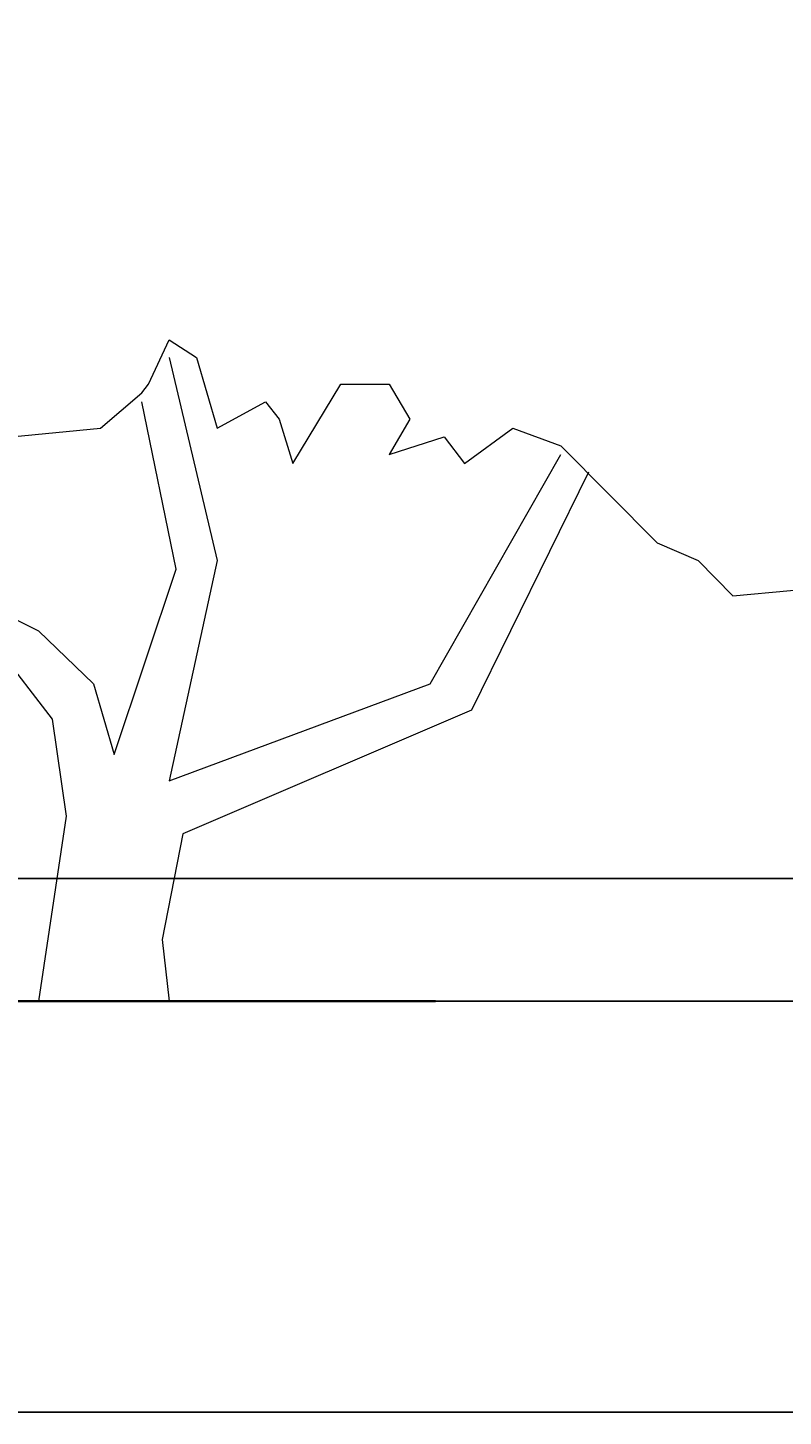
# Model space of a CAD drawing. Units: inches. Extents: x -26 to 776, y -22 to 650.
# Tile 51 of 62: x 642 to 709, y -22 to 102. Entities that reach past the tile are written whole.
import ezdxf

# ---------------------------------------------------------------- set-up
doc = ezdxf.new("R2010")
doc.units = ezdxf.units.IN
doc.header["$MEASUREMENT"] = 0
for name, color, linetype, lineweight in [('A-ANNO-DIMS', 2, 'Continuous', 18), ('C-TOPO', 7, 'Continuous', 35), ('L-PLNT-TREE', 94, 'Continuous', 18)]:
    doc.layers.add(name, color=color, linetype=linetype, lineweight=lineweight)
doc.styles.get("Standard").update_dxf_attribs({"font": 'arial.ttf'})
doc.dimstyles.get("Standard").update_dxf_attribs({"dimtxt": 0.5625, "dimasz": 0.18, "dimexe": 0.18, "dimexo": 0.0625, "dimgap": 0.09, "dimtad": 0, "dimtih": 1, "dimtoh": 1, "dimdec": 4, "dimzin": 0, "dimdsep": 46, "dimlunit": 4, "dimtxsty": 'Standard', "dimcen": 0.09, "dimadec": 0, "dimazin": 0, "dimtfac": 1, "dimtdec": 4, "dimtofl": 0, "dimtmove": 0, "dimatfit": 3, "dimfxl": 1, "dimtolj": 1, "dimtzin": 0, "dimarcsym": 0})

# ---------------------------------------------------------------- blocks, each defined once
blk = doc.blocks.new('Tree - type 3 evergreen elevation')
for points in [[(-1.7254, 35.3906), (3.8821, 35.9436), (6.4701, 38.1555), (6.9014, 38.7085), (8.1954, 41.4734), (9.9208, 40.3674), (11.2148, 35.9436), (14.2341, 37.6025), (15.0968, 36.4966), (15.9595, 33.7317), (18.9789, 38.7085), (21.9982, 38.7085), (23.2922, 36.4966), (21.9982, 34.2847), (25.4489, 35.3906), (26.743, 33.7317), (29.7623, 35.9436), (32.7817, 34.8376), (38.8204, 28.7549), (41.4084, 27.6489), (43.5651, 25.437), (61.6813, 27.0959)], [(8.1954, 40.3674), (11.2148, 27.6489), (8.1954, 13.8245), (24.5862, 19.9072), (32.7817, 34.2847)], [(-9.9208, 28.2019), (0, 23.2251), (3.4507, 19.9072), (4.7447, 15.4834), (8.6267, 27.0959), (6.4701, 37.6025)], [(34.5071, 33.1787), (27.1743, 18.2483), (9.0581, 10.5066), (7.7641, 3.8708), (8.1954, 0)], [(-12.9401, 28.7549), (-2.588, 22.1191), (0.8626, 17.6953), (1.7253, 11.6125), (0, 0)]]:
    blk.add_lwpolyline(points)
blk = doc.blocks.new('*D13')
at = {"layer": 'A-ANNO-DIMS', "color": 0, "lineweight": -2, "transparency": 16777216}
for p, q in [((738.75, 50.79), (738.75, -21.31)), ((11.11, 15.42), (11.11, -21.31)), ((11.29, -21.13), (373.89, -21.13)), ((738.57, -21.13), (375.97, -21.13))]:
    blk.add_line(p, q, dxfattribs=at)
at = {"layer": 'A-ANNO-DIMS', "color": 0, "transparency": 16777216}
for points in [[(11.29, -21.1), (11.29, -21.16), (11.11, -21.13)], [(738.57, -21.1), (738.57, -21.16), (738.75, -21.13)]]:
    blk.add_solid(points, dxfattribs=at)
at = {"layer": 'Defpoints', "color": 0, "transparency": 16777216}
for p in [(738.75, 50.85), (11.11, 15.48), (738.75, -21.13)]:
    blk.add_point(p, dxfattribs=at)
at = {"layer": 'A-ANNO-DIMS', "color": 0, "transparency": 16777216, "insert": (374.93, -21.13), "char_height": 0.562, "attachment_point": 5}
blk.add_mtext('\\A1;727.6', dxfattribs=at)
blk = doc.blocks.new('*D20')
at = {"layer": 'A-ANNO-DIMS', "color": 0, "lineweight": -2, "transparency": 16777216}
for p, q in [((425.81, 455.47), (775.34, 455.47)), ((775.16, 455.29), (775.16, 235.85)), ((775.16, 15.66), (775.16, 235.1)), ((425.81, 15.48), (775.34, 15.48))]:
    blk.add_line(p, q, dxfattribs=at)
at = {"layer": 'A-ANNO-DIMS', "color": 0, "transparency": 16777216}
for points in [[(775.13, 455.29), (775.19, 455.29), (775.16, 455.47)], [(775.13, 15.66), (775.19, 15.66), (775.16, 15.48)]]:
    blk.add_solid(points, dxfattribs=at)
at = {"layer": 'Defpoints', "color": 0, "transparency": 16777216}
for p in [(425.74, 455.47), (775.16, 455.47), (425.74, 15.48)]:
    blk.add_point(p, dxfattribs=at)
at = {"layer": 'A-ANNO-DIMS', "color": 0, "transparency": 16777216, "insert": (775.16, 235.48), "char_height": 0.562, "attachment_point": 5}
blk.add_mtext('\\A1;440', dxfattribs=at)
blk = doc.blocks.new('*D30')
at = {"layer": 'A-ANNO-DIMS', "color": 0, "lineweight": -2, "transparency": 16777216}
for p, q in [((280.68, 144.84), (775.34, 144.84)), ((775.16, 144.66), (775.16, 86.01)), ((775.16, 26.6), (775.16, 85.25)), ((280.68, 26.42), (775.34, 26.42))]:
    blk.add_line(p, q, dxfattribs=at)
at = {"layer": 'A-ANNO-DIMS', "color": 0, "transparency": 16777216}
for points in [[(775.13, 144.66), (775.19, 144.66), (775.16, 144.84)], [(775.13, 26.6), (775.19, 26.6), (775.16, 26.42)]]:
    blk.add_solid(points, dxfattribs=at)
at = {"layer": 'Defpoints', "color": 0, "transparency": 16777216}
for p in [(280.62, 144.84), (775.16, 144.84), (280.62, 26.42)]:
    blk.add_point(p, dxfattribs=at)
at = {"layer": 'A-ANNO-DIMS', "color": 0, "transparency": 16777216, "insert": (775.16, 85.63), "char_height": 0.562, "attachment_point": 5}
blk.add_mtext('\\A1;118.41', dxfattribs=at)
blk = doc.blocks.new('*D38')
at = {"layer": 'A-ANNO-DIMS', "color": 0, "lineweight": -2, "transparency": 16777216}
for p, q in [((280.68, 26.42), (775.34, 26.42)), ((775.16, 26.24), (775.16, 21.33)), ((775.16, 15.66), (775.16, 20.58)), ((289.3, 15.48), (775.34, 15.48))]:
    blk.add_line(p, q, dxfattribs=at)
at = {"layer": 'A-ANNO-DIMS', "color": 0, "transparency": 16777216}
for points in [[(775.13, 26.24), (775.19, 26.24), (775.16, 26.42)], [(775.13, 15.66), (775.19, 15.66), (775.16, 15.48)]]:
    blk.add_solid(points, dxfattribs=at)
at = {"layer": 'Defpoints', "color": 0, "transparency": 16777216}
for p in [(280.62, 26.42), (775.16, 26.42), (289.24, 15.48)]:
    blk.add_point(p, dxfattribs=at)
at = {"layer": 'A-ANNO-DIMS', "color": 0, "transparency": 16777216, "insert": (775.16, 20.95), "char_height": 0.562, "attachment_point": 5}
blk.add_mtext('\\A1;10.942', dxfattribs=at)
blk = doc.blocks.new('*D45')
at = {"layer": 'A-ANNO-DIMS', "color": 0, "lineweight": -2, "transparency": 16777216}
for p, q in [((507.74, 408.64), (775.34, 408.64)), ((775.16, 408.46), (775.16, 212.44)), ((775.16, 15.66), (775.16, 211.68)), ((586, 15.48), (775.34, 15.48))]:
    blk.add_line(p, q, dxfattribs=at)
at = {"layer": 'A-ANNO-DIMS', "color": 0, "transparency": 16777216}
for points in [[(775.13, 408.46), (775.19, 408.46), (775.16, 408.64)], [(775.13, 15.66), (775.19, 15.66), (775.16, 15.48)]]:
    blk.add_solid(points, dxfattribs=at)
at = {"layer": 'Defpoints', "color": 0, "transparency": 16777216}
for p in [(507.68, 408.64), (775.16, 408.64), (585.94, 15.48)]:
    blk.add_point(p, dxfattribs=at)
at = {"layer": 'A-ANNO-DIMS', "color": 0, "transparency": 16777216, "insert": (775.16, 212.06), "char_height": 0.562, "attachment_point": 5}
blk.add_mtext('\\A1;393.16', dxfattribs=at)
blk = doc.blocks.new('*D46')
at = {"layer": 'A-ANNO-DIMS', "color": 0, "lineweight": -2, "transparency": 16777216}
for p, q in [((658.51, 219.03), (775.34, 219.03)), ((775.16, 218.85), (775.16, 117.63)), ((775.16, 15.66), (775.16, 116.88)), ((677.97, 15.48), (775.34, 15.48))]:
    blk.add_line(p, q, dxfattribs=at)
at = {"layer": 'A-ANNO-DIMS', "color": 0, "transparency": 16777216}
for points in [[(775.13, 218.85), (775.19, 218.85), (775.16, 219.03)], [(775.13, 15.66), (775.19, 15.66), (775.16, 15.48)]]:
    blk.add_solid(points, dxfattribs=at)
at = {"layer": 'Defpoints', "color": 0, "transparency": 16777216}
for p in [(658.44, 219.03), (775.16, 219.03), (677.9, 15.48)]:
    blk.add_point(p, dxfattribs=at)
at = {"layer": 'A-ANNO-DIMS', "color": 0, "transparency": 16777216, "insert": (775.16, 117.26), "char_height": 0.562, "attachment_point": 5}
blk.add_mtext('\\A1;203.55', dxfattribs=at)
blk = doc.blocks.new('*D48')
at = {"layer": 'A-ANNO-DIMS', "color": 0, "lineweight": -2, "transparency": 16777216}
for p, q in [((545.03, 67.41), (545.03, 649.86)), ((738.75, 50.91), (738.75, 649.86)), ((545.21, 649.68), (640.88, 649.68)), ((738.57, 649.68), (642.9, 649.68))]:
    blk.add_line(p, q, dxfattribs=at)
at = {"layer": 'A-ANNO-DIMS', "color": 0, "transparency": 16777216}
for points in [[(545.21, 649.71), (545.21, 649.65), (545.03, 649.68)], [(738.57, 649.71), (738.57, 649.65), (738.75, 649.68)]]:
    blk.add_solid(points, dxfattribs=at)
at = {"layer": 'Defpoints', "color": 0, "transparency": 16777216}
for p in [(738.75, 649.68), (545.03, 67.35), (738.75, 50.85)]:
    blk.add_point(p, dxfattribs=at)
at = {"layer": 'A-ANNO-DIMS', "color": 0, "transparency": 16777216, "insert": (641.89, 649.68), "char_height": 0.562, "attachment_point": 5}
blk.add_mtext('\\A1;193.7', dxfattribs=at)

msp = doc.modelspace()

# ---------------------------------------------------------------- linework, layer by layer
at = {"layer": 'C-TOPO'}
msp.add_line((425.7434, 15.4824), (677.9037, 15.4824), dxfattribs=at)

# ---------------------------------------------------------------- block references
at = {"layer": 'L-PLNT-TREE', "xscale": 1.421226385586178, "yscale": 1.421226385586178, "zscale": 1.421226385586178}
msp.add_blockref('Tree - type 3 evergreen elevation', (642.5048, 15.4824), dxfattribs=at)

# ---------------------------------------------------------------- dimensions: what is measured, and where the dimension line sits
at = {"layer": 'A-ANNO-DIMS'}
for base, p1, picture, middle in [((738.7503, 649.6763), (545.0331, 67.3523), '*D48', (641.8917, 649.6763)), ((738.7503, -21.1349), (11.1074, 15.4824), '*D13', (374.9289, -21.1349))]:
    dim = msp.add_linear_dim(base=base, p1=p1, p2=(738.7503, 50.8482), dimstyle='Standard', override={"dimdec": 1, "dimlfac": 1, "dimrnd": 0, "dimzin": 0, "dimdsep": 46, "dimlunit": 2}, dxfattribs=at)
    dim.commit()
    dim.dimension.update_dxf_attribs({"geometry": picture, "text_midpoint": middle})
for base, p1, p2, override, picture, middle in [((775.1553, 455.4717), (425.7434, 15.4824), (425.7434, 455.4717), {"dimdec": 0, "dimlfac": 1, "dimrnd": 0, "dimzin": 0, "dimdsep": 46, "dimlunit": 2}, '*D20', (775.1553, 235.477)), ((775.1553, 408.6389), (585.9354, 15.4824), (507.6759, 408.6389), {"dimdec": 2, "dimlfac": 1, "dimrnd": 0, "dimzin": 0, "dimdsep": 46, "dimlunit": 2}, '*D45', (775.1553, 212.0606)), ((775.1553, 219.0324), (677.9037, 15.4824), (658.4435, 219.0324), {"dimdec": 2, "dimlfac": 1, "dimrnd": 0, "dimzin": 0, "dimdsep": 46, "dimlunit": 2}, '*D46', (775.1553, 117.2574)), ((775.1553, 144.8359), (280.6173, 26.4239), (280.6173, 144.8359), {"dimdec": 2, "dimlfac": 1, "dimrnd": 0, "dimzin": 0, "dimdsep": 46, "dimlunit": 2}, '*D30', (775.1553, 85.6299)), ((775.15535, 26.4239), (289.24236, 15.48237), (280.61732, 26.4239), {"dimdec": 3, "dimlfac": 1, "dimrnd": 0, "dimzin": 0, "dimdsep": 46, "dimlunit": 2}, '*D38', (775.15535, 20.95313))]:
    dim = msp.add_linear_dim(base=base, p1=p1, p2=p2, angle=90, dimstyle='Standard', override=override, dxfattribs=at)
    dim.commit()
    dim.dimension.update_dxf_attribs({"geometry": picture, "text_midpoint": middle})

doc.saveas('drawing.dxf')
